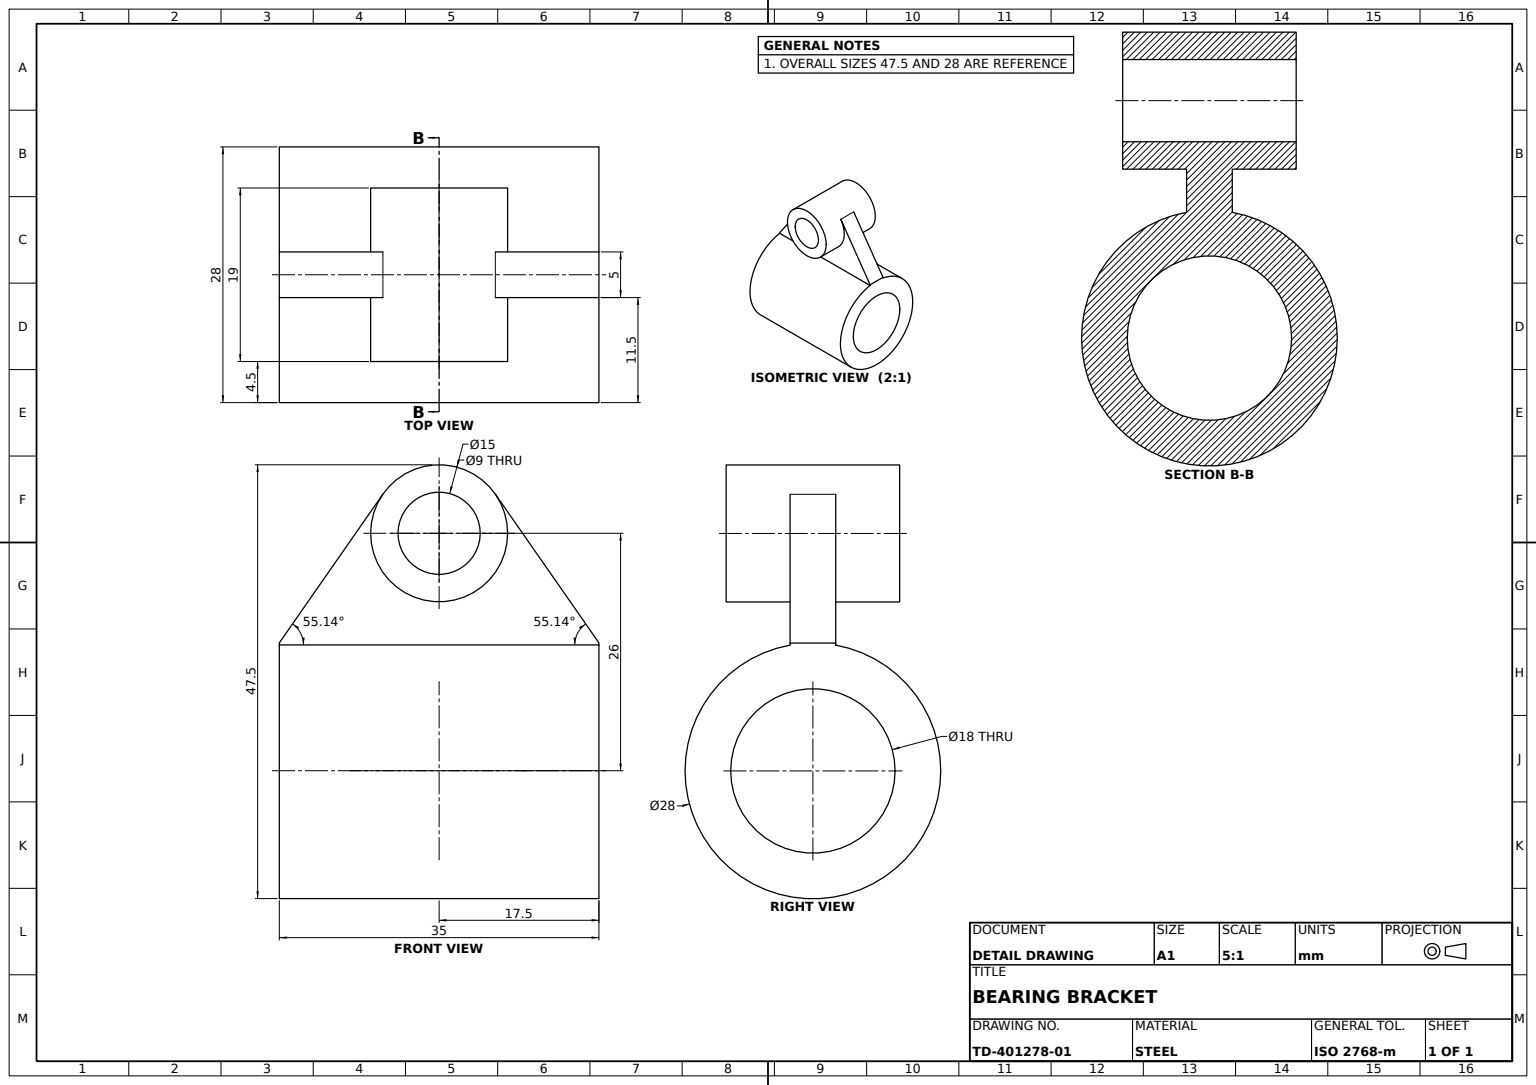
from build123d import *

# Parameters (mm, degrees)
MAIN_BARREL_28_DEPTH      = 17.5
MAIN_BARREL_28_DEPTH_BACK = 17.5
MAIN_BARREL_SKETCH_R      = 14
MAIN_BORE_SKETCH_R        = 9
MAIN_BORE_18_DEPTH        = 41.211938526
UPPER_BOSS_SKETCH_R       = 7.5
UPPER_BOSS_15_DEPTH       = 9.5
UPPER_BORE_SKETCH_R       = 4.5
UPPER_BORE_9_DEPTH        = 45.505617623
CONNECTING_WEB_DEPTH      = 2.5


with BuildPart() as part:
    # Main Barrel Sketch → Main Barrel _28 (new, two sides: drawn at the far end of the back side and taken through both)
    with BuildSketch(Plane.XY.offset(-MAIN_BARREL_28_DEPTH_BACK)):
        Circle(MAIN_BARREL_SKETCH_R)
    extrude(amount=MAIN_BARREL_28_DEPTH + MAIN_BARREL_28_DEPTH_BACK)

    # Main Bore Sketch → Main Bore _18 (cut, through all)
    with BuildSketch(Plane.XY.offset(17.5)):
        Circle(MAIN_BORE_SKETCH_R)
    extrude(amount=-MAIN_BORE_18_DEPTH, mode=Mode.SUBTRACT)



with BuildPart() as body_2:
    # Upper Boss Sketch → Upper Boss _15 (new, symmetric)
    with BuildSketch(Plane(origin=(0, 0, 0), x_dir=(0, 0, -1), z_dir=(1, 0, 0))):
        with Locations((0, 26)):
            Circle(UPPER_BOSS_SKETCH_R)
    extrude(amount=UPPER_BOSS_15_DEPTH, both=True)

    # Upper Bore Sketch → Upper Bore _9 (cut, through all)
    with BuildSketch(Plane(origin=(9.5, 0, 0), x_dir=(0, 0, -1), z_dir=(1, 0, 0))):
        with Locations((0, 26)):
            Circle(UPPER_BORE_SKETCH_R)
    extrude(amount=-UPPER_BORE_9_DEPTH, mode=Mode.SUBTRACT)


with BuildPart() as part_1:
    add(part.part)

    add(body_2.part)  # Connecting Web merges body 2
    # Web Sketch → Connecting Web (add, symmetric)
    with BuildSketch(Plane(origin=(0, 0, 0), x_dir=(0, 0, -1), z_dir=(1, 0, 0))):
        with BuildLine():
            Line((-6.153967777, 30.287036342), (-17.5, 14))
            Line((-17.5, 14), (-17.5, 13))
            Line((-17.5, 13), (17.5, 13))
            Line((17.5, 13), (17.5, 14))
            Line((17.5, 14), (6.153967777, 30.287036342))
            ThreePointArc((6.153967777, 30.287036342), (7.155583775, 28.246691086), (7.5, 26))
            ThreePointArc((7.5, 26), (-2.246691086, 18.844416225), (-6.153967777, 30.287036342))
        make_face()
    extrude(amount=CONNECTING_WEB_DEPTH, both=True)


solid = part_1.part
